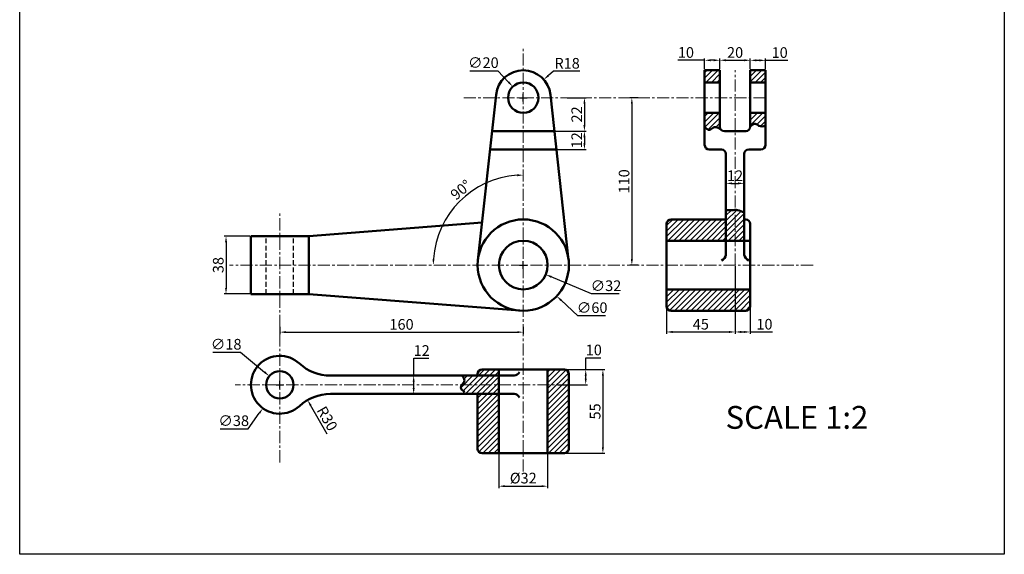
# Model space of a CAD drawing. Units: millimetres. Extents: x 161 to 808, y -21 to 750.
# Tile 1 of 2: x 161 to 808, y -21 to 330. Entities that reach past the tile are written whole.
import ezdxf

# ---------------------------------------------------------------- set-up
doc = ezdxf.new("R2010")
doc.units = ezdxf.units.MM
doc.header["$LTSCALE"] = 0.5
doc.linetypes.add('CENTER', pattern=[50.8, 31.75, -6.35, 6.35, -6.35])
doc.linetypes.add('DASHED', pattern=[19.05, 12.7, -6.35])
for name, color, linetype, lineweight in [('M-CNTR', 1, 'CENTER', 18), ('M-DIMS', 2, 'Continuous', 25), ('M-HATC', 8, 'Continuous', 18), ('M-HIDN', 6, 'DASHED', 25), ('M-OUTL', 7, 'Continuous', 50), ('M-TEXT', 3, 'Continuous', 25), ('M-TTLB', 7, 'Continuous', 25)]:
    doc.layers.add(name, color=color, linetype=linetype, lineweight=lineweight)
doc.styles.get("Standard").update_dxf_attribs({"font": 'arial.ttf'})
doc.dimstyles.new('ISO-25', dxfattribs={"dimtxt": 7, "dimasz": 4, "dimexe": 1.25, "dimexo": 0.625, "dimtad": 1, "dimtoh": 1, "dimtxsty": 'Standard', "dimcen": 2.5, "dimadec": 0, "dimazin": 0, "dimtfac": 1, "dimtofl": 0, "dimtmove": 0, "dimatfit": 3, "dimfxl": 1, "dimarcsym": 0})
pattern_1 = [(45, (-222.2658, 90.1227), (-1.796051, 1.796051), [])]

# ---------------------------------------------------------------- blocks, each defined once
blk = doc.blocks.new('*D20')
at = {"layer": 'Defpoints', "color": 0, "ltscale": 0.5, "transparency": 16777216}
for p in [(313.11, 187.74), (296.76, 149.74), (313.11, 149.74)]:
    blk.add_point(p, dxfattribs=at)
at = {"layer": 'M-DIMS', "color": 0, "lineweight": -2, "ltscale": 0.5, "transparency": 16777216}
for p, q in [((312.49, 187.74), (295.51, 187.74)), ((296.76, 183.74), (296.76, 153.74)), ((312.49, 149.74), (295.51, 149.74))]:
    blk.add_line(p, q, dxfattribs=at)
at = {"layer": 'M-DIMS', "color": 0, "ltscale": 0.5, "transparency": 16777216}
for points in [[(296.1, 183.74), (297.43, 183.74), (296.76, 187.74)], [(296.1, 153.74), (297.43, 153.74), (296.76, 149.74)]]:
    blk.add_solid(points, dxfattribs=at)
at = {"layer": 'M-DIMS', "color": 0, "ltscale": 0.5, "transparency": 16777216, "insert": (292.56, 168.74), "char_height": 7, "attachment_point": 5, "rotation": 90}
blk.add_mtext('38', dxfattribs=at)
blk = doc.blocks.new('*D24')
at = {"layer": 'Defpoints', "color": 0, "ltscale": 0.5, "transparency": 16777216}
for p in [(520.39, 278.74), (512.64, 256.74), (532.3, 256.74)]:
    blk.add_point(p, dxfattribs=at)
at = {"layer": 'M-DIMS', "color": 0, "lineweight": -2, "ltscale": 0.5, "transparency": 16777216}
for p, q in [((521.02, 278.74), (533.55, 278.74)), ((532.3, 274.74), (532.3, 260.74)), ((513.26, 256.74), (533.55, 256.74))]:
    blk.add_line(p, q, dxfattribs=at)
at = {"layer": 'M-DIMS', "color": 0, "ltscale": 0.5, "transparency": 16777216}
for points in [[(531.63, 274.74), (532.96, 274.74), (532.3, 278.74)], [(531.63, 260.74), (532.96, 260.74), (532.3, 256.74)]]:
    blk.add_solid(points, dxfattribs=at)
at = {"layer": 'M-DIMS', "color": 0, "ltscale": 0.5, "transparency": 16777216, "insert": (528.16, 267.74), "char_height": 7, "attachment_point": 5, "rotation": 90}
blk.add_mtext('22', dxfattribs=at)
blk = doc.blocks.new('*D25')
at = {"layer": 'Defpoints', "color": 0, "ltscale": 0.5, "transparency": 16777216}
for p in [(523.4, 256.74), (513.95, 244.74), (532.3, 244.74)]:
    blk.add_point(p, dxfattribs=at)
at = {"layer": 'M-DIMS', "color": 0, "lineweight": -2, "ltscale": 0.5, "transparency": 16777216}
for p, q in [((524.03, 256.74), (533.55, 256.74)), ((532.3, 252.74), (532.3, 248.74)), ((514.58, 244.74), (533.55, 244.74))]:
    blk.add_line(p, q, dxfattribs=at)
at = {"layer": 'M-DIMS', "color": 0, "ltscale": 0.5, "transparency": 16777216}
for points in [[(531.63, 252.74), (532.96, 252.74), (532.3, 256.74)], [(531.63, 248.74), (532.96, 248.74), (532.3, 244.74)]]:
    blk.add_solid(points, dxfattribs=at)
at = {"layer": 'M-DIMS', "color": 0, "ltscale": 0.5, "transparency": 16777216, "insert": (528.16, 250.74), "char_height": 7, "attachment_point": 5, "rotation": 90}
blk.add_mtext('12', dxfattribs=at)
blk = doc.blocks.new('*D26')
at = {"layer": 'Defpoints', "color": 0, "ltscale": 0.5, "transparency": 16777216}
for p in [(568.24, 278.74), (563.47, 168.74), (568.24, 168.74)]:
    blk.add_point(p, dxfattribs=at)
at = {"layer": 'M-DIMS', "color": 0, "lineweight": -2, "ltscale": 0.5, "transparency": 16777216}
for p, q in [((567.62, 278.74), (562.22, 278.74)), ((563.47, 274.74), (563.47, 172.74)), ((567.62, 168.74), (562.22, 168.74))]:
    blk.add_line(p, q, dxfattribs=at)
at = {"layer": 'M-DIMS', "color": 0, "ltscale": 0.5, "transparency": 16777216}
for points in [[(562.81, 274.74), (564.14, 274.74), (563.47, 278.74)], [(562.81, 172.74), (564.14, 172.74), (563.47, 168.74)]]:
    blk.add_solid(points, dxfattribs=at)
at = {"layer": 'M-DIMS', "color": 0, "ltscale": 0.5, "transparency": 16777216, "insert": (559.27, 223.74), "char_height": 7, "attachment_point": 5, "rotation": 90}
blk.add_mtext('110', dxfattribs=at)
blk = doc.blocks.new('*D27')
at = {"layer": 'Defpoints', "color": 0, "ltscale": 0.5, "transparency": 16777216}
for p in [(621.31, 303.32), (611.31, 296.74), (621.31, 296.74)]:
    blk.add_point(p, dxfattribs=at)
at = {"layer": 'M-DIMS', "color": 0, "lineweight": -2, "ltscale": 0.5, "transparency": 16777216}
for p, q in [((611.31, 297.36), (611.31, 304.57)), ((621.31, 297.36), (621.31, 304.57)), ((611.31, 303.32), (593.71, 303.32)), ((617.31, 303.32), (615.31, 303.32))]:
    blk.add_line(p, q, dxfattribs=at)
at = {"layer": 'M-DIMS', "color": 0, "ltscale": 0.5, "transparency": 16777216}
for points in [[(615.31, 303.99), (615.31, 302.65), (611.31, 303.32)], [(617.31, 303.99), (617.31, 302.65), (621.31, 303.32)]]:
    blk.add_solid(points, dxfattribs=at)
at = {"layer": 'M-DIMS', "color": 0, "ltscale": 0.5, "transparency": 16777216, "insert": (599, 307.52), "char_height": 7, "attachment_point": 5}
blk.add_mtext('10', dxfattribs=at)
blk = doc.blocks.new('*D28')
at = {"layer": 'Defpoints', "color": 0, "ltscale": 0.5, "transparency": 16777216}
for p in [(621.31, 303.32), (641.31, 303.32), (641.31, 296.74)]:
    blk.add_point(p, dxfattribs=at)
at = {"layer": 'M-DIMS', "color": 0, "lineweight": -2, "ltscale": 0.5, "transparency": 16777216}
for p, q in [((621.31, 303.95), (621.31, 304.57)), ((641.31, 297.36), (641.31, 304.57)), ((625.31, 303.32), (637.31, 303.32))]:
    blk.add_line(p, q, dxfattribs=at)
at = {"layer": 'M-DIMS', "color": 0, "ltscale": 0.5, "transparency": 16777216}
for points in [[(625.31, 303.99), (625.31, 302.65), (621.31, 303.32)], [(637.31, 303.99), (637.31, 302.65), (641.31, 303.32)]]:
    blk.add_solid(points, dxfattribs=at)
at = {"layer": 'M-DIMS', "color": 0, "ltscale": 0.5, "transparency": 16777216, "insert": (631.31, 307.52), "char_height": 7, "attachment_point": 5}
blk.add_mtext('20', dxfattribs=at)
blk = doc.blocks.new('*D29')
at = {"layer": 'Defpoints', "color": 0, "ltscale": 0.5, "transparency": 16777216}
for p in [(651.31, 303.27), (641.31, 296.74), (651.31, 296.74)]:
    blk.add_point(p, dxfattribs=at)
at = {"layer": 'M-DIMS', "color": 0, "lineweight": -2, "ltscale": 0.5, "transparency": 16777216}
for p, q in [((641.31, 297.36), (641.31, 304.52)), ((651.31, 297.36), (651.31, 304.52)), ((645.31, 303.27), (647.31, 303.27)), ((651.31, 303.27), (665.9, 303.27))]:
    blk.add_line(p, q, dxfattribs=at)
at = {"layer": 'M-DIMS', "color": 0, "ltscale": 0.5, "transparency": 16777216}
for points in [[(645.31, 303.93), (645.31, 302.6), (641.31, 303.27)], [(647.31, 303.93), (647.31, 302.6), (651.31, 303.27)]]:
    blk.add_solid(points, dxfattribs=at)
at = {"layer": 'M-DIMS', "color": 0, "ltscale": 0.5, "transparency": 16777216, "insert": (660.61, 307.47), "char_height": 7, "attachment_point": 5}
blk.add_mtext('10', dxfattribs=at)
blk = doc.blocks.new('*D30')
at = {"layer": 'Defpoints', "color": 0, "ltscale": 0.5, "transparency": 16777216}
for p in [(637.31, 222.42), (625.31, 217), (637.31, 217)]:
    blk.add_point(p, dxfattribs=at)
at = {"layer": 'M-DIMS', "color": 0, "lineweight": -2, "ltscale": 0.5, "transparency": 16777216}
for p, q in [((625.31, 217.62), (625.31, 223.67)), ((629.31, 222.42), (633.31, 222.42)), ((637.31, 217.62), (637.31, 223.67))]:
    blk.add_line(p, q, dxfattribs=at)
at = {"layer": 'M-DIMS', "color": 0, "ltscale": 0.5, "transparency": 16777216}
for points in [[(629.31, 223.09), (629.31, 221.76), (625.31, 222.42)], [(633.31, 223.09), (633.31, 221.76), (637.31, 222.42)]]:
    blk.add_solid(points, dxfattribs=at)
at = {"layer": 'M-DIMS', "color": 0, "ltscale": 0.5, "transparency": 16777216, "insert": (631.31, 226.56), "char_height": 7, "attachment_point": 5}
blk.add_mtext('12', dxfattribs=at)
blk = doc.blocks.new('*D31')
at = {"layer": 'Defpoints', "color": 0, "ltscale": 0.5, "transparency": 16777216}
for p in [(641.31, 157.63), (631.31, 130.32), (641.31, 124.79)]:
    blk.add_point(p, dxfattribs=at)
at = {"layer": 'M-DIMS', "color": 0, "lineweight": -2, "ltscale": 0.5, "transparency": 16777216}
for p, q in [((641.31, 157), (641.31, 123.54)), ((631.31, 129.69), (631.31, 123.54)), ((635.31, 124.79), (637.31, 124.79)), ((641.31, 124.79), (655.9, 124.79))]:
    blk.add_line(p, q, dxfattribs=at)
at = {"layer": 'M-DIMS', "color": 0, "ltscale": 0.5, "transparency": 16777216}
for points in [[(635.31, 125.46), (635.31, 124.12), (631.31, 124.79)], [(637.31, 125.46), (637.31, 124.12), (641.31, 124.79)]]:
    blk.add_solid(points, dxfattribs=at)
at = {"layer": 'M-DIMS', "color": 0, "ltscale": 0.5, "transparency": 16777216, "insert": (650.61, 128.99), "char_height": 7, "attachment_point": 5}
blk.add_mtext('10', dxfattribs=at)
blk = doc.blocks.new('*D32')
at = {"layer": 'Defpoints', "color": 0, "ltscale": 0.5, "transparency": 16777216}
for p in [(586.31, 168.74), (631.31, 168.74), (631.31, 124.79)]:
    blk.add_point(p, dxfattribs=at)
at = {"layer": 'M-DIMS', "color": 0, "lineweight": -2, "ltscale": 0.5, "transparency": 16777216}
for p, q in [((586.31, 168.11), (586.31, 123.54)), ((631.31, 168.11), (631.31, 123.54)), ((590.31, 124.79), (627.31, 124.79))]:
    blk.add_line(p, q, dxfattribs=at)
at = {"layer": 'M-DIMS', "color": 0, "ltscale": 0.5, "transparency": 16777216}
for points in [[(590.31, 125.46), (590.31, 124.12), (586.31, 124.79)], [(627.31, 125.46), (627.31, 124.12), (631.31, 124.79)]]:
    blk.add_solid(points, dxfattribs=at)
at = {"layer": 'M-DIMS', "color": 0, "ltscale": 0.5, "transparency": 16777216, "insert": (608.81, 128.98), "char_height": 7, "attachment_point": 5}
blk.add_mtext('45', dxfattribs=at)
blk = doc.blocks.new('*D33')
at = {"layer": 'Defpoints', "color": 0, "ltscale": 0.5, "transparency": 16777216}
for p in [(425.69, 96.08), (420.09, 84.08), (425.69, 84.08)]:
    blk.add_point(p, dxfattribs=at)
at = {"layer": 'M-DIMS', "color": 0, "lineweight": -2, "ltscale": 0.5, "transparency": 16777216}
for p, q in [((420.09, 96.08), (420.09, 107.56)), ((420.09, 107.56), (430.01, 107.56)), ((425.06, 96.08), (418.84, 96.08)), ((420.09, 88.08), (420.09, 92.08)), ((425.06, 84.08), (418.84, 84.08))]:
    blk.add_line(p, q, dxfattribs=at)
at = {"layer": 'M-DIMS', "color": 0, "ltscale": 0.5, "transparency": 16777216}
for points in [[(419.42, 92.08), (420.75, 92.08), (420.09, 96.08)], [(419.42, 88.08), (420.75, 88.08), (420.09, 84.08)]]:
    blk.add_solid(points, dxfattribs=at)
at = {"layer": 'M-DIMS', "color": 0, "ltscale": 0.5, "transparency": 16777216, "insert": (425.36, 111.7), "char_height": 7, "attachment_point": 5}
blk.add_mtext('12', dxfattribs=at)
blk = doc.blocks.new('*D34')
at = {"layer": 'Defpoints', "color": 0, "ltscale": 0.5, "transparency": 16777216}
for p in [(332.11, 128.78), (492.11, 128.78), (492.11, 124.67)]:
    blk.add_point(p, dxfattribs=at)
at = {"layer": 'M-DIMS', "color": 0, "lineweight": -2, "ltscale": 0.5, "transparency": 16777216}
for p, q in [((332.11, 128.15), (332.11, 123.42)), ((336.11, 124.67), (488.11, 124.67)), ((492.11, 128.15), (492.11, 123.42))]:
    blk.add_line(p, q, dxfattribs=at)
at = {"layer": 'M-DIMS', "color": 0, "ltscale": 0.5, "transparency": 16777216}
for points in [[(336.11, 125.34), (336.11, 124.01), (332.11, 124.67)], [(488.11, 125.34), (488.11, 124.01), (492.11, 124.67)]]:
    blk.add_solid(points, dxfattribs=at)
at = {"layer": 'M-DIMS', "color": 0, "ltscale": 0.5, "transparency": 16777216, "insert": (412.11, 128.87), "char_height": 7, "attachment_point": 5}
blk.add_mtext('160', dxfattribs=at)
blk = doc.blocks.new('*D35')
at = {"layer": 'Defpoints', "color": 0, "ltscale": 0.5, "transparency": 16777216}
for p in [(476.11, 45.08), (508.11, 45.08), (508.11, 23.46)]:
    blk.add_point(p, dxfattribs=at)
at = {"layer": 'M-DIMS', "color": 0, "lineweight": -2, "ltscale": 0.5, "transparency": 16777216}
for p, q in [((476.11, 44.46), (476.11, 22.21)), ((508.11, 44.46), (508.11, 22.21)), ((480.11, 23.46), (504.11, 23.46))]:
    blk.add_line(p, q, dxfattribs=at)
at = {"layer": 'M-DIMS', "color": 0, "ltscale": 0.5, "transparency": 16777216}
for points in [[(480.11, 24.13), (480.11, 22.8), (476.11, 23.46)], [(504.11, 24.13), (504.11, 22.8), (508.11, 23.46)]]:
    blk.add_solid(points, dxfattribs=at)
at = {"layer": 'M-DIMS', "color": 0, "ltscale": 0.5, "transparency": 16777216, "insert": (492.11, 27.86), "char_height": 7, "attachment_point": 5}
blk.add_mtext('%%C32', dxfattribs=at)
blk = doc.blocks.new('*D36')
at = {"layer": 'Defpoints', "color": 0, "ltscale": 0.5, "transparency": 16777216}
for p in [(514.12, 100.08), (514.12, 90.08), (533.15, 90.08)]:
    blk.add_point(p, dxfattribs=at)
at = {"layer": 'M-DIMS', "color": 0, "lineweight": -2, "ltscale": 0.5, "transparency": 16777216}
for p, q in [((533.15, 100.08), (533.15, 107.87)), ((533.15, 107.87), (543.12, 107.87)), ((514.74, 100.08), (534.4, 100.08)), ((533.15, 94.08), (533.15, 96.08)), ((514.74, 90.08), (534.4, 90.08))]:
    blk.add_line(p, q, dxfattribs=at)
at = {"layer": 'M-DIMS', "color": 0, "ltscale": 0.5, "transparency": 16777216}
for points in [[(532.49, 96.08), (533.82, 96.08), (533.15, 100.08)], [(532.49, 94.08), (533.82, 94.08), (533.15, 90.08)]]:
    blk.add_solid(points, dxfattribs=at)
at = {"layer": 'M-DIMS', "color": 0, "ltscale": 0.5, "transparency": 16777216, "insert": (538.45, 112.07), "char_height": 7, "attachment_point": 5}
blk.add_mtext('10', dxfattribs=at)
blk = doc.blocks.new('*D37')
at = {"layer": 'Defpoints', "color": 0, "ltscale": 0.5, "transparency": 16777216}
for p in [(514.12, 100.08), (514.12, 45.08), (544.43, 45.08)]:
    blk.add_point(p, dxfattribs=at)
at = {"layer": 'M-DIMS', "color": 0, "lineweight": -2, "ltscale": 0.5, "transparency": 16777216}
for p, q in [((514.74, 100.08), (545.68, 100.08)), ((544.43, 96.08), (544.43, 49.08)), ((514.74, 45.08), (545.68, 45.08))]:
    blk.add_line(p, q, dxfattribs=at)
at = {"layer": 'M-DIMS', "color": 0, "ltscale": 0.5, "transparency": 16777216}
for points in [[(543.76, 96.08), (545.09, 96.08), (544.43, 100.08)], [(543.76, 49.08), (545.09, 49.08), (544.43, 45.08)]]:
    blk.add_solid(points, dxfattribs=at)
at = {"layer": 'M-DIMS', "color": 0, "ltscale": 0.5, "transparency": 16777216, "insert": (540.24, 72.58), "char_height": 7, "attachment_point": 5, "rotation": 90}
blk.add_mtext('55', dxfattribs=at)
blk = doc.blocks.new('*D38')
at = {"layer": 'Defpoints', "color": 0, "ltscale": 0.5, "transparency": 16777216}
for p in [(477.36, 174.93), (506.86, 162.54)]:
    blk.add_point(p, dxfattribs=at)
at = {"layer": 'M-DIMS', "color": 0, "lineweight": -2, "ltscale": 0.5, "transparency": 16777216}
for p, q in [((489.61, 168.74), (494.61, 168.74)), ((492.11, 166.24), (492.11, 171.24)), ((537.03, 149.87), (510.55, 160.99)), ((555.23, 149.87), (537.03, 149.87))]:
    blk.add_line(p, q, dxfattribs=at)
at = {"layer": 'M-DIMS', "color": 0, "ltscale": 0.5, "transparency": 16777216}
blk.add_solid([(510.81, 161.61), (510.29, 160.38), (506.86, 162.54)], dxfattribs=at)
at = {"layer": 'M-DIMS', "color": 0, "ltscale": 0.5, "transparency": 16777216, "insert": (546.44, 154.27), "char_height": 7, "attachment_point": 5}
blk.add_mtext('∅32', dxfattribs=at)
blk = doc.blocks.new('*D39')
at = {"layer": 'Defpoints', "color": 0, "ltscale": 0.5, "transparency": 16777216}
for p in [(470.13, 189.16), (514.09, 148.32)]:
    blk.add_point(p, dxfattribs=at)
at = {"layer": 'M-DIMS', "color": 0, "lineweight": -2, "ltscale": 0.5, "transparency": 16777216}
for p, q in [((489.61, 168.74), (494.61, 168.74)), ((492.11, 166.24), (492.11, 171.24)), ((527.93, 135.46), (517.02, 145.6)), ((546.18, 135.46), (527.93, 135.46))]:
    blk.add_line(p, q, dxfattribs=at)
at = {"layer": 'M-DIMS', "color": 0, "ltscale": 0.5, "transparency": 16777216}
blk.add_solid([(517.48, 146.08), (516.57, 145.11), (514.09, 148.32)], dxfattribs=at)
at = {"layer": 'M-DIMS', "color": 0, "ltscale": 0.5, "transparency": 16777216, "insert": (537.37, 139.85), "char_height": 7, "attachment_point": 5}
blk.add_mtext('∅60', dxfattribs=at)
blk = doc.blocks.new('*D40')
at = {"layer": 'Defpoints', "color": 0, "ltscale": 0.5, "transparency": 16777216}
for p in [(343.23, 105.49), (320.99, 74.68)]:
    blk.add_point(p, dxfattribs=at)
at = {"layer": 'M-DIMS', "color": 0, "lineweight": -2, "ltscale": 0.5, "transparency": 16777216}
for p, q in [((332.11, 87.58), (332.11, 92.58)), ((329.61, 90.08), (334.61, 90.08)), ((311.25, 61.18), (318.65, 71.44)), ((292.97, 61.18), (311.25, 61.18))]:
    blk.add_line(p, q, dxfattribs=at)
at = {"layer": 'M-DIMS', "color": 0, "ltscale": 0.5, "transparency": 16777216}
blk.add_solid([(318.11, 71.83), (319.19, 71.04), (320.99, 74.68)], dxfattribs=at)
at = {"layer": 'M-DIMS', "color": 0, "ltscale": 0.5, "transparency": 16777216, "insert": (301.8, 65.58), "char_height": 7, "attachment_point": 5}
blk.add_mtext('∅38', dxfattribs=at)
blk = doc.blocks.new('*D41')
at = {"layer": 'Defpoints', "color": 0, "ltscale": 0.5, "transparency": 16777216}
for p in [(325.18, 95.82), (339.05, 84.35)]:
    blk.add_point(p, dxfattribs=at)
at = {"layer": 'M-DIMS', "color": 0, "lineweight": -2, "ltscale": 0.5, "transparency": 16777216}
for p, q in [((288.02, 111.43), (306.31, 111.43)), ((306.31, 111.43), (322.1, 98.37)), ((332.11, 87.58), (332.11, 92.58)), ((329.61, 90.08), (334.61, 90.08))]:
    blk.add_line(p, q, dxfattribs=at)
at = {"layer": 'M-DIMS', "color": 0, "ltscale": 0.5, "transparency": 16777216}
blk.add_solid([(322.52, 98.88), (321.67, 97.86), (325.18, 95.82)], dxfattribs=at)
at = {"layer": 'M-DIMS', "color": 0, "ltscale": 0.5, "transparency": 16777216, "insert": (296.85, 115.83), "char_height": 7, "attachment_point": 5}
blk.add_mtext('∅18', dxfattribs=at)
blk = doc.blocks.new('*D42')
at = {"layer": 'Defpoints', "color": 0, "ltscale": 0.5, "transparency": 16777216}
for p in [(350.35, 80.07), (365.35, 54.08)]:
    blk.add_point(p, dxfattribs=at)
at = {"layer": 'M-DIMS', "color": 0, "lineweight": -2, "ltscale": 0.5, "transparency": 16777216}
blk.add_line((363.33, 57.59), (352.35, 76.6), dxfattribs=at)
at = {"layer": 'M-DIMS', "color": 0, "ltscale": 0.5, "transparency": 16777216}
blk.add_solid([(352.93, 76.93), (351.78, 76.27), (350.35, 80.07)], dxfattribs=at)
at = {"layer": 'M-DIMS', "color": 0, "ltscale": 0.5, "transparency": 16777216, "insert": (362.48, 67.46), "char_height": 7, "attachment_point": 5, "rotation": 300}
blk.add_mtext('R30', dxfattribs=at)
blk = doc.blocks.new('*D43')
at = {"layer": 'Defpoints', "color": 0, "ltscale": 0.5, "transparency": 16777216}
for p in [(492.11, 310.92), (440.9, 198.31), (299.1, 168.74), (682.53, 168.74), (492.11, 33.13)]:
    blk.add_point(p, dxfattribs=at)
at = {"layer": 'M-DIMS', "color": 0, "lineweight": -2, "ltscale": 0.5, "transparency": 16777216}
blk.add_arc((492.11, 168.74), 59.14, 93.87624, 176.12376, dxfattribs=at)
at = {"layer": 'M-DIMS', "color": 0, "ltscale": 0.5, "transparency": 16777216}
for points in [[(488.09, 228.41), (488.14, 227.07), (492.11, 227.87)], [(433.78, 172.71), (432.45, 172.76), (432.98, 168.74)]]:
    blk.add_solid(points, dxfattribs=at)
at = {"layer": 'M-DIMS', "color": 0, "ltscale": 0.5, "transparency": 16777216, "insert": (451.68, 217.49), "char_height": 7, "attachment_point": 5, "rotation": 39.67429}
blk.add_mtext('90°', dxfattribs=at)
blk = doc.blocks.new('*D44')
at = {"layer": 'Defpoints', "color": 0, "ltscale": 0.5, "transparency": 16777216}
for p in [(505.61, 290.64), (492.11, 278.74)]:
    blk.add_point(p, dxfattribs=at)
at = {"layer": 'M-DIMS', "color": 0, "lineweight": -2, "ltscale": 0.5, "transparency": 16777216}
for p, q in [((511.94, 296.22), (508.61, 293.29)), ((529.3, 296.22), (511.94, 296.22)), ((489.61, 278.74), (494.61, 278.74)), ((492.11, 276.24), (492.11, 281.24))]:
    blk.add_line(p, q, dxfattribs=at)
at = {"layer": 'M-DIMS', "color": 0, "ltscale": 0.5, "transparency": 16777216}
blk.add_solid([(508.17, 293.79), (509.05, 292.79), (505.61, 290.64)], dxfattribs=at)
at = {"layer": 'M-DIMS', "color": 0, "ltscale": 0.5, "transparency": 16777216, "insert": (520.93, 300.42), "char_height": 7, "attachment_point": 5}
blk.add_mtext('R18', dxfattribs=at)
blk = doc.blocks.new('*D45')
at = {"layer": 'Defpoints', "color": 0, "ltscale": 0.5, "transparency": 16777216}
for p in [(485.23, 285.99), (499, 271.49)]:
    blk.add_point(p, dxfattribs=at)
at = {"layer": 'M-DIMS', "color": 0, "lineweight": -2, "ltscale": 0.5, "transparency": 16777216}
for p, q in [((457.06, 296.44), (475.31, 296.44)), ((475.31, 296.44), (482.47, 288.89)), ((489.61, 278.74), (494.61, 278.74)), ((492.11, 276.24), (492.11, 281.24))]:
    blk.add_line(p, q, dxfattribs=at)
at = {"layer": 'M-DIMS', "color": 0, "ltscale": 0.5, "transparency": 16777216}
blk.add_solid([(482.96, 289.35), (481.99, 288.43), (485.23, 285.99)], dxfattribs=at)
at = {"layer": 'M-DIMS', "color": 0, "ltscale": 0.5, "transparency": 16777216, "insert": (465.87, 300.83), "char_height": 7, "attachment_point": 5}
blk.add_mtext('∅20', dxfattribs=at)

msp = doc.modelspace()

# ---------------------------------------------------------------- hatches: boundary and pattern name
at = {"layer": 'M-HATC', "ltscale": 0.5}
h = msp.add_hatch(dxfattribs=at)
h.set_pattern_fill('ANSI31', color=256, scale=0.8)
h.set_pattern_definition(pattern_1)
h.paths.add_polyline_path([(625.309, 198.738), (589.309, 198.738, 0.4142136), (586.309, 195.738), (586.309, 184.738), (625.309, 184.738)])
h.paths.add_polyline_path([(631.309, 152.738), (586.309, 152.738), (586.309, 141.738, 0.4142136), (589.309, 138.738), (631.309, 138.738)])
h.paths.add_polyline_path([(641.309, 152.738), (631.309, 152.738), (631.309, 138.738), (638.309, 138.738, 0.4142136), (641.309, 141.738)])
h.paths.add_polyline_path([(651.309, 296.738), (641.309, 296.738), (641.309, 288.738), (651.309, 288.738)])
h.paths.add_polyline_path([(621.309, 296.738), (611.309, 296.738), (611.309, 288.738), (621.309, 288.738)])
edge = h.paths.add_edge_path()
edge.add_line((621.309, 268.738), (611.309, 268.738))
edge.add_line((611.309, 268.738), (611.309, 259.49))
edge.add_spline(control_points=[(611.309, 259.49), (612.39, 258.471), (614.344, 256.631), (616.787, 259.531), (619.842, 259.304), (621.35, 258.219), (622.188, 257.617)], knot_values=[0, 0, 0, 0, 3.6850041, 6.6612595, 9.1100922, 12.1739581, 12.1739581, 12.1739581, 12.1739581], degree=3, periodic=0)
edge.add_arc((624.309, 259.738), 3, 180, 225, ccw=False)
edge.add_line((621.309, 259.738), (621.309, 268.738))
edge = h.paths.add_edge_path()
edge.add_line((651.309, 268.738), (641.309, 268.738))
edge.add_line((641.309, 268.738), (641.309, 259.738))
edge.add_spline(control_points=[(641.309, 259.738), (642.418, 260.792), (644.335, 262.615), (647.356, 259.398), (649.815, 259.93), (651.309, 260.253)], knot_values=[0, 0, 0, 0, 3.8050822, 6.581159, 10.8817081, 10.8817081, 10.8817081, 10.8817081], degree=3, periodic=0)
edge.add_line((651.309, 260.253), (651.309, 268.738))
h = msp.add_hatch(dxfattribs=at)
h.set_pattern_fill('ANSI31', color=256, scale=0.8)
h.set_pattern_definition(pattern_1)
edge = h.paths.add_edge_path()
edge.add_spline(control_points=[(637.309, 203.291), (635.859, 203.976), (633.921, 204.891), (631.838, 204.965), (631.309, 204.959)], knot_values=[5.9853917, 5.9853917, 5.9853917, 5.9853917, 10.6917803, 12.2745408, 12.2745408, 12.2745408, 12.2745408], degree=3, periodic=0)
edge.add_line((631.309, 204.959), (631.309, 184.738))
edge.add_line((631.309, 184.738), (637.309, 184.738))
edge.add_line((637.309, 184.738), (637.309, 203.291))
edge = h.paths.add_edge_path()
edge.add_spline(control_points=[(631.309, 204.959), (630.624, 204.951), (628.604, 204.808), (626.616, 204.848), (625.309, 204.874)], knot_values=[0, 0, 0, 0, 2.0504074, 5.9853917, 5.9853917, 5.9853917, 5.9853917], degree=3, periodic=0)
edge.add_line((625.309, 204.874), (625.309, 184.738))
edge.add_line((625.309, 184.738), (631.309, 184.738))
edge.add_line((631.309, 184.738), (631.309, 204.959))
h = msp.add_hatch(dxfattribs=at)
h.set_pattern_fill('ANSI31', color=256, scale=0.8)
h.set_pattern_definition(pattern_1)
edge = h.paths.add_edge_path()
edge.add_line((476.113, 90.085), (451.71, 90.085))
edge.add_spline(control_points=[(451.71, 90.085), (451.023, 89.043), (450.713, 86.597), (453.603, 86.116), (453.298, 84.78), (453.138, 84.085)], knot_values=[6.8824551, 6.8824551, 6.8824551, 6.8824551, 10.2677691, 11.9168314, 13.7069863, 13.7069863, 13.7069863, 13.7069863], degree=3, periodic=0)
edge.add_line((453.138, 84.085), (476.113, 84.085))
edge.add_line((476.113, 84.085), (476.113, 90.085))
edge = h.paths.add_edge_path()
edge.add_line((476.113, 96.085), (451.962, 96.085))
edge.add_spline(control_points=[(451.962, 96.085), (452.475, 95.401), (453.368, 94.211), (453.522, 91.609), (452.204, 90.833), (451.71, 90.085)], knot_values=[0, 0, 0, 0, 2.554042, 4.4500115, 6.8824551, 6.8824551, 6.8824551, 6.8824551], degree=3, periodic=0)
edge.add_line((451.71, 90.085), (476.113, 90.085))
edge.add_line((476.113, 90.085), (476.113, 96.085))
h.paths.add_polyline_path([(476.113, 100.085), (465.113, 100.085, 0.4142136), (462.113, 97.085), (462.113, 96.085), (476.113, 96.085)])
h.paths.add_polyline_path([(476.113, 84.085), (462.113, 84.085), (462.113, 48.085, 0.4142136), (465.113, 45.085), (476.113, 45.085)])
h.paths.add_polyline_path([(522.113, 90.085), (508.113, 90.085), (508.113, 45.085), (519.113, 45.085, 0.4142136), (522.113, 48.085)])
h.paths.add_polyline_path([(522.113, 97.085, 0.4142136), (519.113, 100.085), (508.113, 100.085), (508.113, 90.085), (522.113, 90.085)])

# ---------------------------------------------------------------- linework, layer by layer
at = {"layer": 'M-CNTR', "ltscale": 0.5}
for p, q in [((492.113, 33.13), (492.113, 310.925)), ((631.309, 130.318), (631.309, 296.738)), ((453.001, 278.738), (651.309, 278.738)), ((332.113, 39.132), (332.113, 203.23)), ((682.528, 168.738), (299.096, 168.738)), ((522.113, 90.085), (302.771, 90.085))]:
    msp.add_line(p, q, dxfattribs=at)
at = {"layer": 'M-HIDN', "ltscale": 0.5}
for p, q in [((323.113, 149.738), (323.113, 187.738)), ((341.113, 149.738), (341.113, 187.738))]:
    msp.add_line(p, q, dxfattribs=at)
at = {"layer": 'M-OUTL', "ltscale": 0.5}
for p, q in [((611.309, 296.738), (621.309, 296.738)), ((611.309, 247.738), (611.309, 296.738)), ((621.309, 259.738), (621.309, 296.738)), ((641.309, 259.738), (641.309, 296.738)), ((641.309, 296.738), (651.309, 296.738)), ((651.309, 247.738), (651.309, 296.738)), ((611.309, 288.738), (621.309, 288.738)), ((641.309, 288.738), (651.309, 288.738)), ((474.22, 280.702), (462.292, 172.011)), ((510.005, 280.702), (521.934, 172.011)), ((611.309, 268.738), (621.309, 268.738)), ((641.309, 268.738), (651.309, 268.738)), ((471.59, 256.738), (512.635, 256.738)), ((624.309, 256.738), (638.309, 256.738)), ((470.273, 244.738), (513.952, 244.738)), ((614.309, 244.738), (622.309, 244.738)), ((625.309, 241.738), (625.309, 175.549)), ((637.309, 241.738), (637.309, 175.549)), ((640.309, 244.738), (648.309, 244.738)), ((465.001, 196.698), (351.113, 187.738)), ((586.309, 195.738), (586.309, 141.738)), ((625.309, 198.738), (589.309, 198.738)), ((638.309, 198.738), (637.309, 198.738)), ((641.309, 141.738), (641.309, 195.738)), ((332.113, 187.738), (313.113, 187.738)), ((313.113, 187.738), (313.113, 149.738)), ((351.113, 187.738), (332.113, 187.738)), ((351.113, 149.738), (351.113, 187.738)), ((586.309, 184.738), (641.309, 184.738)), ((313.113, 149.738), (351.113, 149.738)), ((489.76, 138.83), (351.113, 149.738)), ((586.309, 152.738), (641.309, 152.738)), ((589.309, 138.738), (638.309, 138.738)), ((462.113, 96.085), (462.113, 97.085)), ((465.113, 100.085), (492.113, 100.085)), ((476.113, 45.085), (476.113, 100.085)), ((492.113, 100.085), (519.113, 100.085)), ((508.113, 45.085), (508.113, 100.085)), ((522.113, 97.085), (522.113, 48.085)), ((486.019, 96.085), (365.354, 96.085)), ((486.019, 84.085), (365.354, 84.085)), ((462.113, 48.085), (462.113, 84.085)), ((519.113, 45.085), (465.113, 45.085))]:
    msp.add_line(p, q, dxfattribs=at)
for centre, radius in [((492.113, 278.738), 10), ((492.113, 168.738), 30), ((492.113, 168.738), 16), ((332.113, 90.085), 9)]:
    msp.add_circle(centre, radius, dxfattribs=at)
for centre, radius, start, end in [((492.113, 278.738), 18, 6.262913, 173.737087), ((624.309, 259.738), 3, 180, 270), ((638.309, 259.738), 3, 270, 0), ((614.309, 247.738), 3, 180, 270), ((648.309, 247.738), 3, 270, 0), ((622.309, 241.738), 3, 0, 90), ((640.309, 241.738), 3, 90, 180), ((589.309, 195.738), 3, 90, 180), ((638.309, 195.738), 3, 0, 90), ((620.548, 176.221), 4.808, 291.968407, 351.968407), ((642.07, 176.221), 4.808, 188.031593, 248.031593), ((589.309, 141.738), 3, 180, 270), ((638.309, 141.738), 3, 270, 0), ((332.113, 90.085), 19, 47.281355, 312.718645), ((365.354, 126.085), 30, 227.281355, 270), ((465.113, 97.085), 3, 90, 180), ((485.562, 100.976), 4.913, 275.333418, 327.802007), ((519.113, 97.085), 3, 0, 90), ((365.354, 54.085), 30, 90, 132.718645), ((485.562, 79.193), 4.913, 32.197993, 84.666582), ((465.113, 48.085), 3, 180, 270), ((519.113, 48.085), 3, 270, 0)]:
    msp.add_arc(centre, radius, start, end, dxfattribs=at)
for points, knots in [([(611.309, 259.49), (612.39, 258.471), (614.344, 256.631), (616.787, 259.531), (619.842, 259.304), (621.35, 258.219), (622.188, 257.617)], [0, 0, 0, 0, 3.6850041, 6.6612595, 9.1100922, 12.1739581, 12.1739581, 12.1739581, 12.1739581]), ([(641.309, 259.738), (642.418, 260.792), (644.335, 262.615), (647.356, 259.398), (649.815, 259.93), (651.309, 260.253)], [0, 0, 0, 0, 3.8050822, 6.581159, 10.8817081, 10.8817081, 10.8817081, 10.8817081]), ([(625.309, 204.874), (626.616, 204.848), (629.13, 204.797), (633.29, 205.19), (635.859, 203.976), (637.309, 203.291)], [0, 0, 0, 0, 3.9349844, 7.5681523, 12.2745408, 12.2745408, 12.2745408, 12.2745408]), ([(451.962, 96.085), (452.475, 95.401), (453.368, 94.211), (453.522, 91.609), (451.173, 90.225), (450.713, 86.597), (453.603, 86.116), (453.298, 84.78), (453.138, 84.085)], [0, 0, 0, 0, 2.554042, 4.4500115, 6.8824551, 10.2677691, 11.9168314, 13.7069863, 13.7069863, 13.7069863, 13.7069863])]:
    msp.add_open_spline(points, degree=3, knots=knots, dxfattribs=at)
at = {"layer": 'M-TTLB', "ltscale": 0.5}
msp.add_lwpolyline([(161.16, 749.71), (808.244, 749.71), (808.244, -21.293), (161.16, -21.293)], close=True, dxfattribs=at)

# ---------------------------------------------------------------- texts
at = {"layer": 'M-TEXT', "ltscale": 0.5, "insert": (625.039, 76.162), "char_height": 15, "attachment_point": 1}
msp.add_mtext_dynamic_manual_height_columns('SCALE 1:2', width=111.67008, gutter_width=12.5, heights=[0], dxfattribs=at)

# ---------------------------------------------------------------- dimensions: what is measured, and where the dimension line sits
at = {"layer": 'M-DIMS', "ltscale": 0.5}
dim = msp.add_angular_dim_2l(base=(440.899, 198.306), line1=((492.113, 33.13), (492.113, 310.925)), line2=((682.528, 168.738), (299.096, 168.738)), dimstyle='ISO-25', override={"dimclrd": 0, "dimclre": 0, "dimclrt": 0}, dxfattribs=at)
dim.commit()
dim.dimension.update_dxf_attribs({"geometry": '*D43', "text_midpoint": (454.359, 214.254), "dimtype": 162})
dim = msp.add_linear_dim(base=(621.309, 303.32), p1=(611.309, 296.738), p2=(621.309, 296.738), dimstyle='ISO-25', override={"dimclrd": 0, "dimclre": 0, "dimclrt": 0}, dxfattribs=at)
dim.commit()
dim.dimension.update_dxf_attribs({"geometry": '*D27', "text_midpoint": (599.004, 303.32), "dimtype": 160})
for base, p1, p2, picture, middle in [((641.309, 303.32), (621.309, 303.32), (641.309, 296.738), '*D28', (631.309, 307.519)), ((651.309, 303.266), (641.309, 296.738), (651.309, 296.738), '*D29', (660.606, 307.465)), ((637.309, 222.423), (625.309, 216.995), (637.309, 216.995), '*D30', (631.309, 226.562)), ((631.309, 124.791), (586.309, 168.738), (631.309, 168.738), '*D32', (608.809, 128.975)), ((641.309, 124.791), (631.309, 130.318), (641.309, 157.628), '*D31', (650.606, 128.99)), ((492.113, 124.675), (332.113, 128.777), (492.113, 128.777), '*D34', (412.113, 128.874))]:
    dim = msp.add_linear_dim(base=base, p1=p1, p2=p2, dimstyle='ISO-25', override={"dimclrd": 0, "dimclre": 0, "dimclrt": 0}, dxfattribs=at)
    dim.commit()
    dim.dimension.update_dxf_attribs({"geometry": picture, "text_midpoint": middle})
for p1, p2, picture, middle in [((498.998, 271.486), (485.227, 285.99), '*D45', (465.871, 296.438)), ((470.134, 189.157), (514.091, 148.319), '*D39', (537.367, 135.459)), ((477.361, 174.934), (506.864, 162.542), '*D38', (546.445, 149.871)), ((339.048, 84.348), (325.178, 95.821), '*D41', (296.852, 111.432)), ((343.233, 105.491), (320.993, 74.678), '*D40', (301.799, 61.185))]:
    dim = msp.add_diameter_dim_2p(p1=p1, p2=p2, dimstyle='ISO-25', override={"dimclrd": 0, "dimclre": 0, "dimclrt": 0}, dxfattribs=at)
    dim.commit()
    dim.dimension.update_dxf_attribs({"geometry": picture, "text_midpoint": middle, "dimtype": 163})
for center, mpoint, picture, middle in [((492.113, 278.738), (505.612, 290.645), '*D44', (520.931, 296.222)), ((365.354, 54.085), (350.354, 80.065), '*D42', (358.842, 65.363))]:
    dim = msp.add_radius_dim(center=center, mpoint=mpoint, dimstyle='ISO-25', override={"dimclrd": 0, "dimclre": 0, "dimclrt": 0}, dxfattribs=at)
    dim.commit()
    dim.dimension.update_dxf_attribs({"geometry": picture, "text_midpoint": middle, "dimtype": 164})
for base, p1, p2, picture, middle in [((532.298, 256.738), (520.392, 278.738), (512.635, 256.738), '*D24', (528.159, 267.738)), ((563.474, 168.738), (568.243, 278.738), (568.243, 168.738), '*D26', (559.275, 223.738)), ((532.298, 244.738), (523.404, 256.738), (513.952, 244.738), '*D25', (528.159, 250.738)), ((296.762, 149.738), (313.113, 187.738), (313.113, 149.738), '*D20', (292.56, 168.738)), ((544.426, 45.085), (514.117, 100.085), (514.117, 45.085), '*D37', (540.241, 72.585))]:
    dim = msp.add_linear_dim(base=base, p1=p1, p2=p2, angle=90, dimstyle='ISO-25', override={"dimclrd": 0, "dimclre": 0, "dimclrt": 0}, dxfattribs=at)
    dim.commit()
    dim.dimension.update_dxf_attribs({"geometry": picture, "text_midpoint": middle})
for base, p1, p2, picture, middle in [((533.153, 90.085), (514.117, 100.085), (514.117, 90.085), '*D36', (538.45, 107.872)), ((420.088, 84.085), (425.686, 96.085), (425.686, 84.085), '*D33', (425.361, 107.564))]:
    dim = msp.add_linear_dim(base=base, p1=p1, p2=p2, angle=90, dimstyle='ISO-25', override={"dimclrd": 0, "dimclre": 0, "dimclrt": 0}, dxfattribs=at)
    dim.commit()
    dim.dimension.update_dxf_attribs({"geometry": picture, "text_midpoint": middle, "dimtype": 160})
dim = msp.add_linear_dim(base=(508.113, 23.462), p1=(476.113, 45.085), p2=(508.113, 45.085), text='%%C<>', dimstyle='ISO-25', override={"dimclrd": 0, "dimclre": 0, "dimclrt": 0}, dxfattribs=at)
dim.commit()
dim.dimension.update_dxf_attribs({"geometry": '*D35', "text_midpoint": (492.113, 23.462), "dimtype": 160})

doc.saveas('drawing.dxf')
